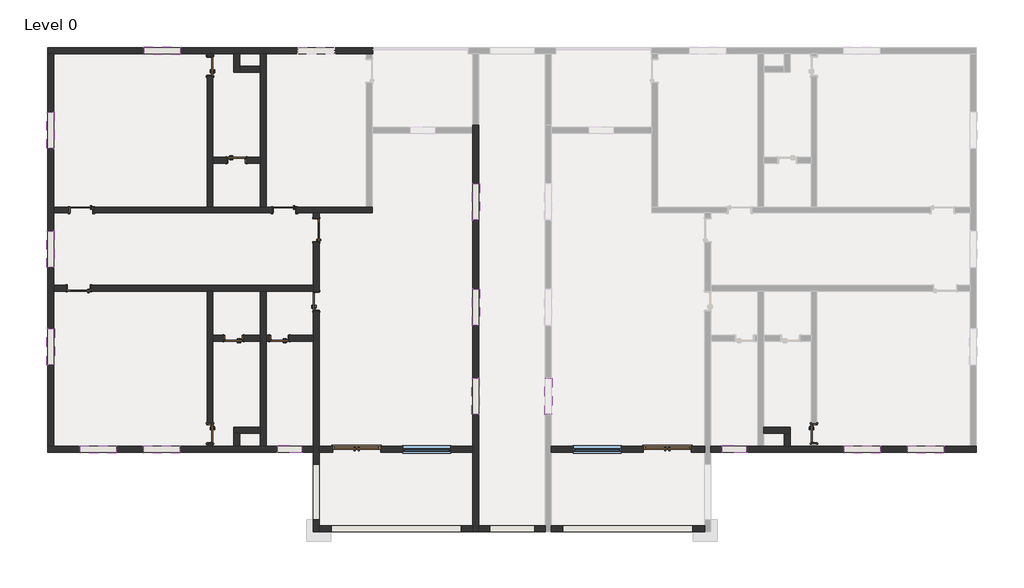
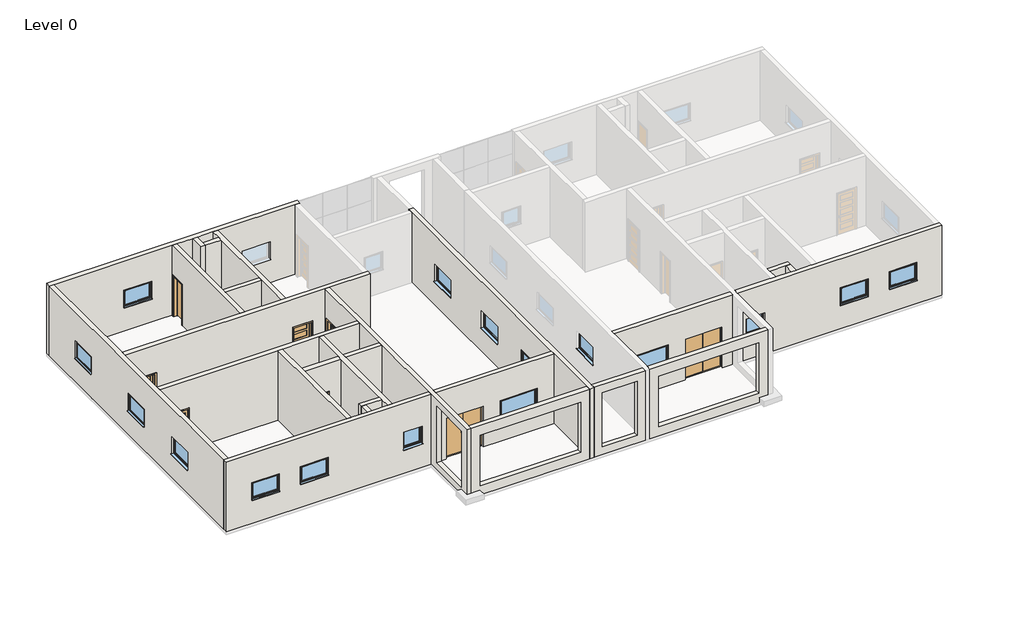
# One storey, part 1 of 2: 25 walls, 16 windows, 13 doors.
# Revit data of these elements (continued)
# Element 48 (IfcWindow, "Windows_Sgl_Plain : 1360x910mm")
#   Mark = "38"
#   Phase Created = New Construction
#   Materials on its faces: "Window Frame", "Glass"
# Element 49 (IfcWindow, "Windows_Sgl_Plain : 1360x910mm")
#   Mark = "39"
#   Phase Created = New Construction
#   Materials on its faces: "Window Frame", "Glass"
# Element 50 (IfcWindow, "Windows_Sgl_Plain : 1360x910mm")
#   Mark = "43"
#   Phase Created = New Construction
#   Materials on its faces: "Window Frame", "Glass"
# Element 51 (IfcWindow, "Windows_Sgl_Plain : 1810x1210mm")
#   Mark = "18"
#   Phase Created = New Construction
#   Materials on its faces: "Window Frame", "Glass"
# Element 52 (IfcWindow, "Windows_Sgl_Plain : 1810x1210mm")
#   Mark = "33"
#   Phase Created = New Construction
#   Materials on its faces: "Window Frame", "Glass"
# Element 53 (IfcWindow, "Windows_Sgl_Plain : 910x910mm")
#   Mark = "31"
#   Phase Created = New Construction
#   Materials on its faces: "Window Frame", "Glass"
# Element 54 (IfcWindow, "Windows_Sgl_Plain : 910x910mm")
#   Mark = "44"
#   Phase Created = New Construction
#   Materials on its faces: "Window Frame", "Glass"
# Materials
#   "Cherry": class "Wood", colour RGB 226 177 128, transparency 0, Description = "Prunus Serotina", Cost = 0
#   "Aluminum": class "Metal", colour RGB 247 247 247, transparency 0, Description = "Aluminum 6061", Cost = 0
#   "Door - Panel": class "Wood", colour RGB 210 159 95, transparency 0, Keynote = "L20", Cost = 0
#   "Door - Frame/Mullion": class "Wood", colour RGB 212 179 113, transparency 0, Keynote = "L20", Cost = 0
#   "Door - Handle": colour RGB 0 0 0, transparency 0, Keynote = "P21", Cost = 0
#   "Door - Frame/Mullion (1)": class "Wood", colour RGB 212 179 113, transparency 0, Keynote = "L20", Cost = 0
#   "Door - Architrave": class "Wood", colour RGB 154 90 5, transparency 0, Keynote = "P20", Cost = 0
#   "Concrete, Precast": class "Concrete", colour RGB 130 132 119, transparency 0, Description = "Precast concrete", Cost = 0
#   "Window Frame": colour RGB 249 249 249, transparency 0, Keynote = "L10", Cost = 0
#   "Glass": class "Glass", colour RGB 0 128 192, transparency 0.9, Description = "Soda Lime Glass", Cost = 0
# Room at (11943.408, 10849.65) mm, phase "New Construction", upper level "Level 0", upper offset 4000 mm, lower offset 0 mm
#   Number = "5"
# Room at (1131.525, 9084.445) mm, phase "New Construction", upper level "Level 0", upper offset 4000 mm, lower offset 0 mm
#   Number = "1"
#   Name = "BED ROOM"
# Room at (4937.749, 10309.076) mm, phase "New Construction", upper level "Level 0", upper offset 4000 mm, lower offset 0 mm
#   Number = "2"
#   Name = "BATHROOM"
# Room at (8082.021, 9084.445) mm, phase "New Construction", upper level "Level 0", upper offset 4000 mm, lower offset 0 mm
#   Number = "3"
#   Name = "KITCHEN"
# Room at (4937.749, 7098.589) mm, phase "New Construction", upper level "Level 0", upper offset 4000 mm, lower offset 0 mm
#   Number = "4"
#   Name = "CLOSET"
# Room at (10931.408, 2244.274) mm, phase "New Construction", upper level "Level 0", upper offset 4000 mm, lower offset 0 mm
#   Number = "6"
#   Name = "LIVING ROOM"
# Room at (2786.405, 4836.919) mm, phase "New Construction", upper level "Level 0", upper offset 4000 mm, lower offset 0 mm
#   Number = "7"
#   Name = "LOBBY"
# Room at (4937.749, -569.022) mm, phase "New Construction", upper level "Level 0", upper offset 4000 mm, lower offset 0 mm
#   Number = "11"
#   Name = "BATHROOM"
# Room at (7107.021, -569.022) mm, phase "New Construction", upper level "Level 0", upper offset 4000 mm, lower offset 0 mm
#   Number = "12"
#   Name = "BATHROOM"
# Room at (10931.408, -4430.409) mm, phase "New Construction", upper level "Level 0", upper offset 4000 mm, lower offset 0 mm
#   Number = "13"
#   Name = "SIT OUT"
# Room at (11943.408, 7485.409) mm, phase "New Construction", upper level "Level 0", upper offset 4000 mm, lower offset 0 mm
#   Number = "14"
#   Name = "DINING"
# Room at (29570.821, 9084.445) mm, phase "New Construction", upper level "Level 0", upper offset 4000 mm, lower offset 0 mm
#   Number = "15"
#   Name = "BED ROOM"
# Room at (25764.597, 10309.076) mm, phase "New Construction", upper level "Level 0", upper offset 4000 mm, lower offset 0 mm
#   Number = "16"
#   Name = "BATHROOM"
# Room at (25764.597, 7098.589) mm, phase "New Construction", upper level "Level 0", upper offset 4000 mm, lower offset 0 mm
#   Number = "18"
#   Name = "CLOSET"
# Room at (18758.939, 10849.65) mm, phase "New Construction", upper level "Level 0", upper offset 4000 mm, lower offset 0 mm
#   Number = "19"
# Room at (19770.939, 2244.274) mm, phase "New Construction", upper level "Level 0", upper offset 4000 mm, lower offset 0 mm
#   Number = "20"
#   Name = "LIVING ROOM"
# Room at (27915.941, 4836.919) mm, phase "New Construction", upper level "Level 0", upper offset 4000 mm, lower offset 0 mm
#   Number = "21"
#   Name = "LOBBY"
# Room at (29570.821, 0) mm, phase "New Construction", upper level "Level 0", upper offset 4000 mm, lower offset 0 mm
#   Number = "22"
#   Name = "BED ROOM"
# Room at (25764.597, 2244.274) mm, phase "New Construction", upper level "Level 0", upper offset 4000 mm, lower offset 0 mm
#   Number = "23"
#   Name = "CLOSET"
# Room at (23595.325, 2244.274) mm, phase "New Construction", upper level "Level 0", upper offset 4000 mm, lower offset 0 mm
#   Number = "24"
#   Name = "LOBBY"
# Room at (25764.597, -569.022) mm, phase "New Construction", upper level "Level 0", upper offset 4000 mm, lower offset 0 mm
#   Number = "25"
#   Name = "BATHROOM"
# Room at (23595.325, -569.022) mm, phase "New Construction", upper level "Level 0", upper offset 4000 mm, lower offset 0 mm
#   Number = "26"
#   Name = "BATHROOM"
# Room at (19770.939, -4430.409) mm, phase "New Construction", upper level "Level 0", upper offset 4000 mm, lower offset 0 mm
#   Number = "27"
#   Name = "SIT OUT"
# Room at (18758.939, 7485.409) mm, phase "New Construction", upper level "Level 0", upper offset 4000 mm, lower offset 0 mm
#   Number = "28"
#   Name = "DINING"
# Room at (22620.325, 9084.445) mm, phase "New Construction", upper level "Level 0", upper offset 4000 mm, lower offset 0 mm
#   Number = "17"
#   Name = "KITCHEN"
# Room at (1131.525, 0) mm, phase "New Construction", upper level "Level 0", upper offset 4000 mm, lower offset 0 mm
#   Number = "8"
#   Name = "BED ROOM"
# Room at (4937.749, 2244.274) mm, phase "New Construction", upper level "Level 0", upper offset 4000 mm, lower offset 0 mm
#   Number = "9"
#   Name = "CLOSET"
# Room at (7107.021, 2244.274) mm, phase "New Construction", upper level "Level 0", upper offset 4000 mm, lower offset 0 mm
#   Number = "10"
#   Name = "LOBBY"
